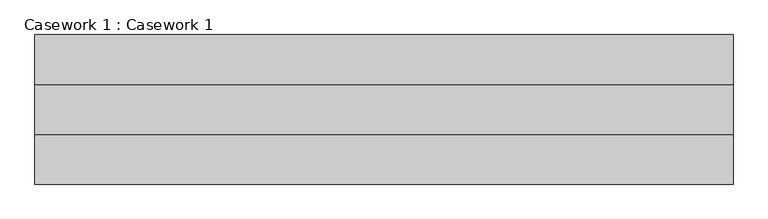
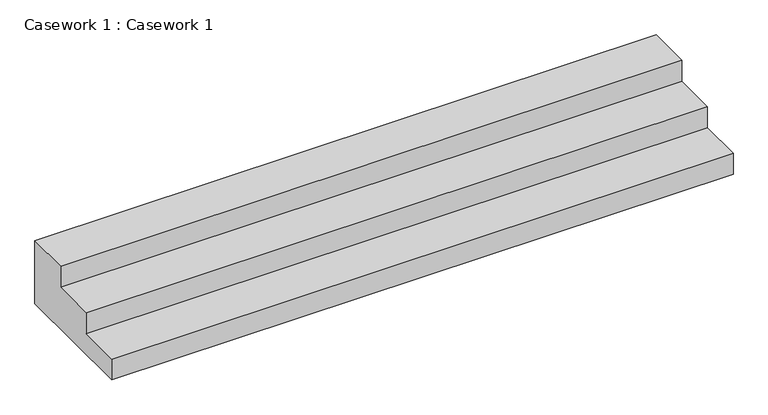
"""IFC4 building model written with IfcOpenShell, lengths in millimetres: furniture geometry, Casework 1 : Casework 1."""

from ifc_helpers import new_model, si_unit, frame, origin, place, context, project, spatial, polyline, outline, extrude, source, transform, mapped, element, save


def casework_1_casework_1_95f3130b(model_context):
    return source(origin(), model_context, "Body", "SweptSolid", [
        extrude(outline(polyline([(-4046.1831926, 1854.5808949), (-3741.3831926, 1854.5808949), (-3741.3831926, 1397.3808949), (-4655.7831926, 1397.3808949), (-4655.7831926, 1549.7808949), (-4350.9831926, 1549.7808949), (-4350.9831926, 1702.1808949), (-4046.1831926, 1702.1808949), (-4046.1831926, 1854.5808949)])), frame((-9376.0719122, 0.0, 0.0), z_axis=(1.0, 0.0, 0.0), x_axis=(0.0, 1.0, 0.0)), (0.0, 0.0, 1.0), 4267.2),
    ])


if __name__ == "__main__":
    model = new_model("IFC4")
    model_context = context("Model", 3, world=origin())
    ifc_project = project(units=[si_unit("LENGTHUNIT", "METRE", prefix="MILLI")], contexts=[model_context])
    site = spatial("IfcSite", under=ifc_project)
    building = spatial("IfcBuilding", under=site)
    placement = place(None, origin())
    casework_1_casework_1_shape = casework_1_casework_1_95f3130b(model_context)
    element("IfcFurniture", 1, ObjectType="Casework 1 : Casework 1", at=placement, inside=building, context=model_context, shape_type="MappedRepresentation", body=[
        mapped(casework_1_casework_1_shape, transform((0.0, 0.0, 0.0), x_axis=(1.0, 0.0, 0.0), y_axis=(0.0, 1.0, 0.0), z_axis=(0.0, 0.0, 1.0))),
    ])
    save(model, "model.ifc")
